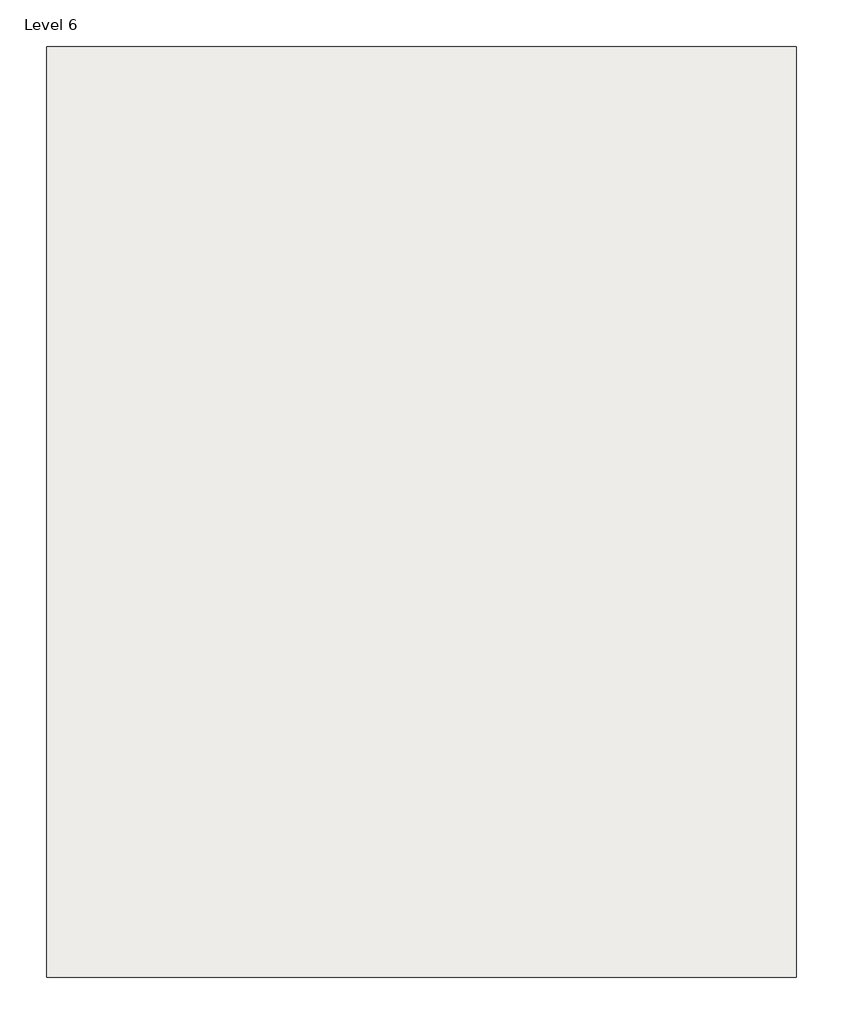
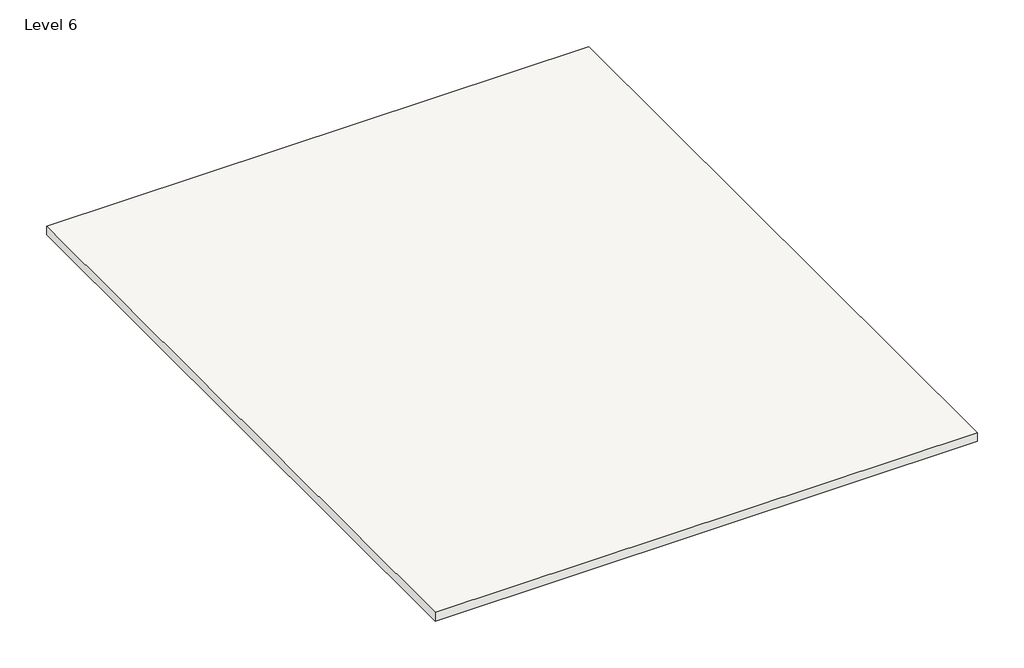
# One storey, incomplete: 1 roof.
"""IFC4 building model written with IfcOpenShell, lengths in millimetres."""

from ifc_helpers import new_model, si_unit, frame, origin, place, context, project, spatial, polyline, outline, extrude, element, save

model = new_model("IFC4")

# Units and contexts
model_context = context("Model", 3, world=origin())
ifc_project = project(units=[si_unit("LENGTHUNIT", "METRE", prefix="MILLI")], contexts=[model_context])

# Site, building, storey
site = spatial("IfcSite", under=ifc_project)
building = spatial("IfcBuilding", under=site)
storey = spatial("IfcBuildingStorey", under=building, Name="Level 6", Elevation=15240.0)

# Roof
placement = place(None, origin())
element("IfcRoof", 1, ObjectType="Generic - 12\"", at=placement, inside=storey, context=model_context, shape_type="SweptSolid", body=[
    extrude(outline(polyline([(660.4, 15087.6), (9499.6, 15087.6), (9499.6, 4114.8), (660.4, 4114.8), (660.4, 15087.6)])), frame((0.0, 0.0, 15240.0), z_axis=(0.0, 0.0, 1.0), x_axis=(1.0, 0.0, 0.0)), (0.0, 0.0, 1.0), 152.4),
])

save(model, "model.ifc")

# Revit data of these elements
# Type "Generic - 12\""
#   Assembly Code = "B1020"
#   Layers, outside or top first: 0' - 6" no material (function 1)
# Element 1 (IfcRoof, "Generic - 12\"")
#   built-in parameter 1001705 = 50.5 (stored number, unit not read)
#   built-in parameter 1001710 = 33615
#   Phase Created = New Construction
#   Materials on its faces: "Textile - Linen, Smooth", "Default Roof"
# Materials
#   "Textile - Linen, Smooth": colour RGB 249 239 230, transparency 0
#   "Default Roof": colour RGB 88 101 114, transparency 0, Cost = 0
